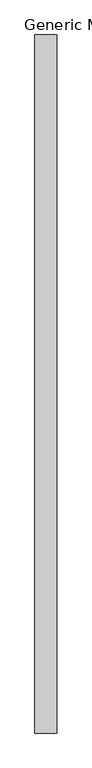
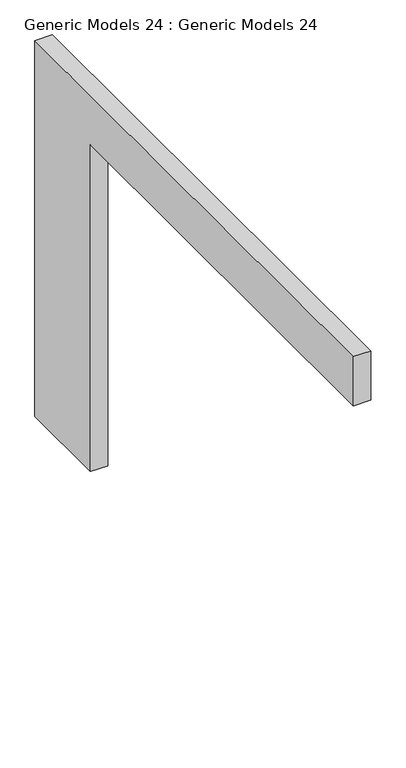
"""IFC4 building model written with IfcOpenShell, lengths in millimetres: proxy geometry, Generic Models 24 : Generic Models 24."""

from ifc_helpers import new_model, si_unit, frame, origin, place, context, project, spatial, polyline, outline, extrude, source, transform, mapped, element, save


def generic_models_24_generic_models_24_dfffe260(model_context):
    return source(origin(), model_context, "Body", "SweptSolid", [
        extrude(outline(polyline([(4970.6155883, 7318.375), (4970.6155883, 6400.8), (4970.6155883, 304.8), (3274.6511874, 304.8), (3274.6511874, 6400.8), (-4757.5844117, 6400.8), (-4757.5844117, 7318.375), (4970.6155883, 7318.375)])), frame((66.1413992, 0.0, 0.0), z_axis=(1.0, 0.0, 0.0), x_axis=(0.0, 1.0, 0.0)), (0.0, 0.0, 1.0), 304.8),
    ])


if __name__ == "__main__":
    model = new_model("IFC4")
    model_context = context("Model", 3, world=origin())
    ifc_project = project(units=[si_unit("LENGTHUNIT", "METRE", prefix="MILLI")], contexts=[model_context])
    site = spatial("IfcSite", under=ifc_project)
    building = spatial("IfcBuilding", under=site)
    placement = place(None, origin())
    generic_models_24_generic_models_24_shape = generic_models_24_generic_models_24_dfffe260(model_context)
    element("IfcBuildingElementProxy", 1, Name="Generic Models 24 : Generic Models 24", ObjectType="Generic Models 24 : Generic Models 24", at=placement, inside=building, context=model_context, shape_type="MappedRepresentation", body=[
        mapped(generic_models_24_generic_models_24_shape, transform((0.0, 0.0, 0.0), x_axis=(1.0, 0.0, 0.0), y_axis=(0.0, 1.0, 0.0), z_axis=(0.0, 0.0, 1.0))),
    ])
    save(model, "model.ifc")

# Revit data of these elements
# Element 1 (IfcBuildingElementProxy, "Generic Models 24 : Generic Models 24")
#   Materials on its faces: "OFF WHITE COLOUR"
# Materials
#   "OFF WHITE COLOUR": class "Generic", colour RGB 120 120 120, transparency 0, Cost = 0
